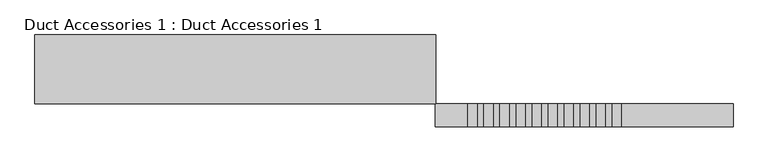
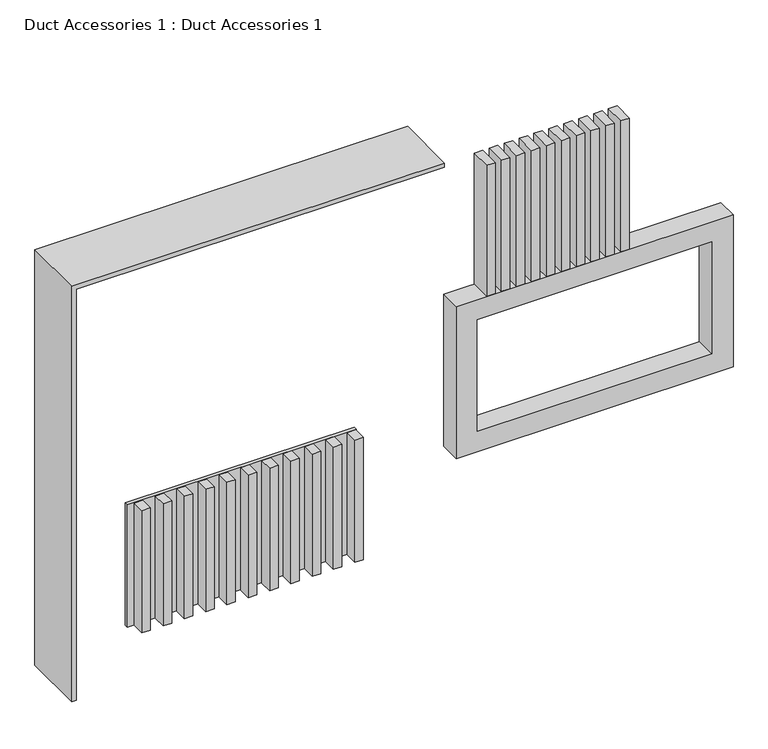
"""IFC4 building model written with IfcOpenShell, lengths in millimetres: damper geometry, Duct Accessories 1 : Duct Accessories 1."""

from ifc_helpers import new_model, si_unit, frame, origin, place, context, project, spatial, polyline, outline, extrude, source, transform, mapped, element, save


def duct_accessories_1_duct_accessories_1_02249294(model_context):
    return source(origin(), model_context, "Body", "SweptSolid", [
        extrude(outline(polyline([(-10129.0101268, -5235.4994609), (-10250.9301268, -5235.4994609), (-10250.9301268, -5048.1296146), (-10129.0101268, -5048.1296146), (-10129.0101268, -5235.4994609)])), frame((0.0, 0.0, 3000.0), z_axis=(0.0, 0.0, 1.0), x_axis=(1.0, 0.0, 0.0)), (0.0, 0.0, 1.0), 1850.0),
        extrude(outline(polyline([(-9824.2101268, -5235.4994609), (-9946.1301268, -5235.4994609), (-9946.1301268, -5048.1296146), (-9824.2101268, -5048.1296146), (-9824.2101268, -5235.4994609)])), frame((0.0, 0.0, 3000.0), z_axis=(0.0, 0.0, 1.0), x_axis=(1.0, 0.0, 0.0)), (0.0, 0.0, 1.0), 1850.0),
        extrude(outline(polyline([(-9519.4101268, -5235.4994609), (-9641.3301268, -5235.4994609), (-9641.3301268, -5048.1296146), (-9519.4101268, -5048.1296146), (-9519.4101268, -5235.4994609)])), frame((0.0, 0.0, 3000.0), z_axis=(0.0, 0.0, 1.0), x_axis=(1.0, 0.0, 0.0)), (0.0, 0.0, 1.0), 1850.0),
        extrude(outline(polyline([(-9214.6101268, -5235.4994609), (-9336.5301268, -5235.4994609), (-9336.5301268, -5048.1296146), (-9214.6101268, -5048.1296146), (-9214.6101268, -5235.4994609)])), frame((0.0, 0.0, 3000.0), z_axis=(0.0, 0.0, 1.0), x_axis=(1.0, 0.0, 0.0)), (0.0, 0.0, 1.0), 1850.0),
        extrude(outline(polyline([(-8909.8101268, -5235.4994609), (-9031.7301268, -5235.4994609), (-9031.7301268, -5048.1296146), (-8909.8101268, -5048.1296146), (-8909.8101268, -5235.4994609)])), frame((0.0, 0.0, 3000.0), z_axis=(0.0, 0.0, 1.0), x_axis=(1.0, 0.0, 0.0)), (0.0, 0.0, 1.0), 1850.0),
        extrude(outline(polyline([(-8605.0101268, -5235.4994609), (-8726.9301268, -5235.4994609), (-8726.9301268, -5048.1296146), (-8605.0101268, -5048.1296146), (-8605.0101268, -5235.4994609)])), frame((0.0, 0.0, 3000.0), z_axis=(0.0, 0.0, 1.0), x_axis=(1.0, 0.0, 0.0)), (0.0, 0.0, 1.0), 1850.0),
        extrude(outline(polyline([(-8300.2101268, -5235.4994609), (-8422.1301268, -5235.4994609), (-8422.1301268, -5048.1296146), (-8300.2101268, -5048.1296146), (-8300.2101268, -5235.4994609)])), frame((0.0, 0.0, 3000.0), z_axis=(0.0, 0.0, 1.0), x_axis=(1.0, 0.0, 0.0)), (0.0, 0.0, 1.0), 1850.0),
        extrude(outline(polyline([(-7995.4101268, -5235.4994609), (-8117.3301268, -5235.4994609), (-8117.3301268, -5048.1296146), (-7995.4101268, -5048.1296146), (-7995.4101268, -5235.4994609)])), frame((0.0, 0.0, 3000.0), z_axis=(0.0, 0.0, 1.0), x_axis=(1.0, 0.0, 0.0)), (0.0, 0.0, 1.0), 1850.0),
        extrude(outline(polyline([(-7690.6101268, -5235.4994609), (-7812.5301268, -5235.4994609), (-7812.5301268, -5048.1296146), (-7690.6101268, -5048.1296146), (-7690.6101268, -5235.4994609)])), frame((0.0, 0.0, 3000.0), z_axis=(0.0, 0.0, 1.0), x_axis=(1.0, 0.0, 0.0)), (0.0, 0.0, 1.0), 1850.0),
        extrude(outline(polyline([(-7385.8101268, -5235.4994609), (-7507.7301268, -5235.4994609), (-7507.7301268, -5048.1296146), (-7385.8101268, -5048.1296146), (-7385.8101268, -5235.4994609)])), frame((0.0, 0.0, 3000.0), z_axis=(0.0, 0.0, 1.0), x_axis=(1.0, 0.0, 0.0)), (0.0, 0.0, 1.0), 1850.0),
        extrude(outline(polyline([(-7081.0101268, -5235.4994609), (-7202.9301268, -5235.4994609), (-7202.9301268, -5048.1296146), (-7081.0101268, -5048.1296146), (-7081.0101268, -5235.4994609)])), frame((0.0, 0.0, 3000.0), z_axis=(0.0, 0.0, 1.0), x_axis=(1.0, 0.0, 0.0)), (0.0, 0.0, 1.0), 1850.0),
        extrude(outline(polyline([(-7067.4667042, -5040.4296146), (-10344.0667042, -5040.4296146), (-10344.0667042, -4990.9296146), (-7067.4667042, -4990.9296146), (-7067.4667042, -5040.4296146)])), frame((0.0, 0.0, 3000.0), z_axis=(0.0, 0.0, 1.0), x_axis=(1.0, 0.0, 0.0)), (0.0, 0.0, 1.0), 1850.0),
        extrude(outline(polyline([(2850.0, -11637.4667042), (2850.0, -11576.5067042), (9070.24, -11576.5067042), (9070.24, -6306.9843842), (9131.2, -6306.9843842), (9131.2, -11637.4667042), (2850.0, -11637.4667042)])), frame((0.0, -5905.3296146, 0.0), z_axis=(0.0, 1.0, 0.0), x_axis=(0.0, 0.0, 1.0)), (0.0, 0.0, 1.0), 914.4),
        extrude(outline(polyline([(-5758.3443842, -6210.1296146), (-5880.2643842, -6210.1296146), (-5880.2643842, -5905.3296146), (-5758.3443842, -5905.3296146), (-5758.3443842, -6210.1296146)])), frame((0.0, 0.0, 7150.0), z_axis=(0.0, 0.0, 1.0), x_axis=(1.0, 0.0, 0.0)), (0.0, 0.0, 1.0), 1981.2),
        extrude(outline(polyline([(-5544.9843842, -6210.1296146), (-5666.9043842, -6210.1296146), (-5666.9043842, -5905.3296146), (-5544.9843842, -5905.3296146), (-5544.9843842, -6210.1296146)])), frame((0.0, 0.0, 7150.0), z_axis=(0.0, 0.0, 1.0), x_axis=(1.0, 0.0, 0.0)), (0.0, 0.0, 1.0), 1981.2),
        extrude(outline(polyline([(-5331.6243842, -6210.1296146), (-5453.5443842, -6210.1296146), (-5453.5443842, -5905.3296146), (-5331.6243842, -5905.3296146), (-5331.6243842, -6210.1296146)])), frame((0.0, 0.0, 7150.0), z_axis=(0.0, 0.0, 1.0), x_axis=(1.0, 0.0, 0.0)), (0.0, 0.0, 1.0), 1981.2),
        extrude(outline(polyline([(-5118.2643842, -6210.1296146), (-5240.1843842, -6210.1296146), (-5240.1843842, -5905.3296146), (-5118.2643842, -5905.3296146), (-5118.2643842, -6210.1296146)])), frame((0.0, 0.0, 7150.0), z_axis=(0.0, 0.0, 1.0), x_axis=(1.0, 0.0, 0.0)), (0.0, 0.0, 1.0), 1981.2),
        extrude(outline(polyline([(-4904.9043842, -6210.1296146), (-5026.8243842, -6210.1296146), (-5026.8243842, -5905.3296146), (-4904.9043842, -5905.3296146), (-4904.9043842, -6210.1296146)])), frame((0.0, 0.0, 7150.0), z_axis=(0.0, 0.0, 1.0), x_axis=(1.0, 0.0, 0.0)), (0.0, 0.0, 1.0), 1981.2),
        extrude(outline(polyline([(-4691.5443842, -6210.1296146), (-4813.4643842, -6210.1296146), (-4813.4643842, -5905.3296146), (-4691.5443842, -5905.3296146), (-4691.5443842, -6210.1296146)])), frame((0.0, 0.0, 7150.0), z_axis=(0.0, 0.0, 1.0), x_axis=(1.0, 0.0, 0.0)), (0.0, 0.0, 1.0), 1981.2),
        extrude(outline(polyline([(-4478.1843842, -6210.1296146), (-4600.1043842, -6210.1296146), (-4600.1043842, -5905.3296146), (-4478.1843842, -5905.3296146), (-4478.1843842, -6210.1296146)])), frame((0.0, 0.0, 7150.0), z_axis=(0.0, 0.0, 1.0), x_axis=(1.0, 0.0, 0.0)), (0.0, 0.0, 1.0), 1981.2),
        extrude(outline(polyline([(-4264.8243842, -6210.1296146), (-4386.7443842, -6210.1296146), (-4386.7443842, -5905.3296146), (-4264.8243842, -5905.3296146), (-4264.8243842, -6210.1296146)])), frame((0.0, 0.0, 7150.0), z_axis=(0.0, 0.0, 1.0), x_axis=(1.0, 0.0, 0.0)), (0.0, 0.0, 1.0), 1981.2),
        extrude(outline(polyline([(-4051.4643842, -6210.1296146), (-4173.3843842, -6210.1296146), (-4173.3843842, -5905.3296146), (-4051.4643842, -5905.3296146), (-4051.4643842, -6210.1296146)])), frame((0.0, 0.0, 7150.0), z_axis=(0.0, 0.0, 1.0), x_axis=(1.0, 0.0, 0.0)), (0.0, 0.0, 1.0), 1981.2),
        extrude(outline(polyline([(-3838.1043842, -6210.1296146), (-3960.0243842, -6210.1296146), (-3960.0243842, -5905.3296146), (-3838.1043842, -5905.3296146), (-3838.1043842, -6210.1296146)])), frame((0.0, 0.0, 7150.0), z_axis=(0.0, 0.0, 1.0), x_axis=(1.0, 0.0, 0.0)), (0.0, 0.0, 1.0), 1981.2),
        extrude(outline(polyline([(4850.0, -6315.8667042), (4850.0, -2353.4667042), (7150.0, -2353.4667042), (7150.0, -6315.8667042), (4850.0, -6315.8667042)]), holes=[polyline([(6845.2, -6011.0667042), (6845.2, -2658.2667042), (5154.8, -2658.2667042), (5154.8, -6011.0667042), (6845.2, -6011.0667042)])]), frame((0.0, -6210.1296146, 0.0), z_axis=(0.0, 1.0, 0.0), x_axis=(0.0, 0.0, 1.0)), (0.0, 0.0, 1.0), 304.8),
    ])


if __name__ == "__main__":
    model = new_model("IFC4")
    model_context = context("Model", 3, world=origin())
    ifc_project = project(units=[si_unit("LENGTHUNIT", "METRE", prefix="MILLI")], contexts=[model_context])
    site = spatial("IfcSite", under=ifc_project)
    building = spatial("IfcBuilding", under=site)
    placement = place(None, origin())
    duct_accessories_1_duct_accessories_1_shape = duct_accessories_1_duct_accessories_1_02249294(model_context)
    element("IfcDamper", 1, ObjectType="Duct Accessories 1 : Duct Accessories 1", at=placement, inside=building, context=model_context, shape_type="MappedRepresentation", body=[
        mapped(duct_accessories_1_duct_accessories_1_shape, transform((0.0, 0.0, 0.0), x_axis=(1.0, 0.0, 0.0), y_axis=(0.0, 1.0, 0.0), z_axis=(0.0, 0.0, 1.0))),
    ])
    save(model, "model.ifc")

# Revit data of these elements
# Element 1 (IfcDamper, "Duct Accessories 1 : Duct Accessories 1")
#   Materials on its faces: "Clad - White", "Wood - Stained"
# Materials
#   "Clad - White": class "Wood", colour RGB 242 242 238, transparency 0, Cost = 0
#   "Wood - Stained": class "Wood", colour RGB 224 178 126, transparency 0, Cost = 0
